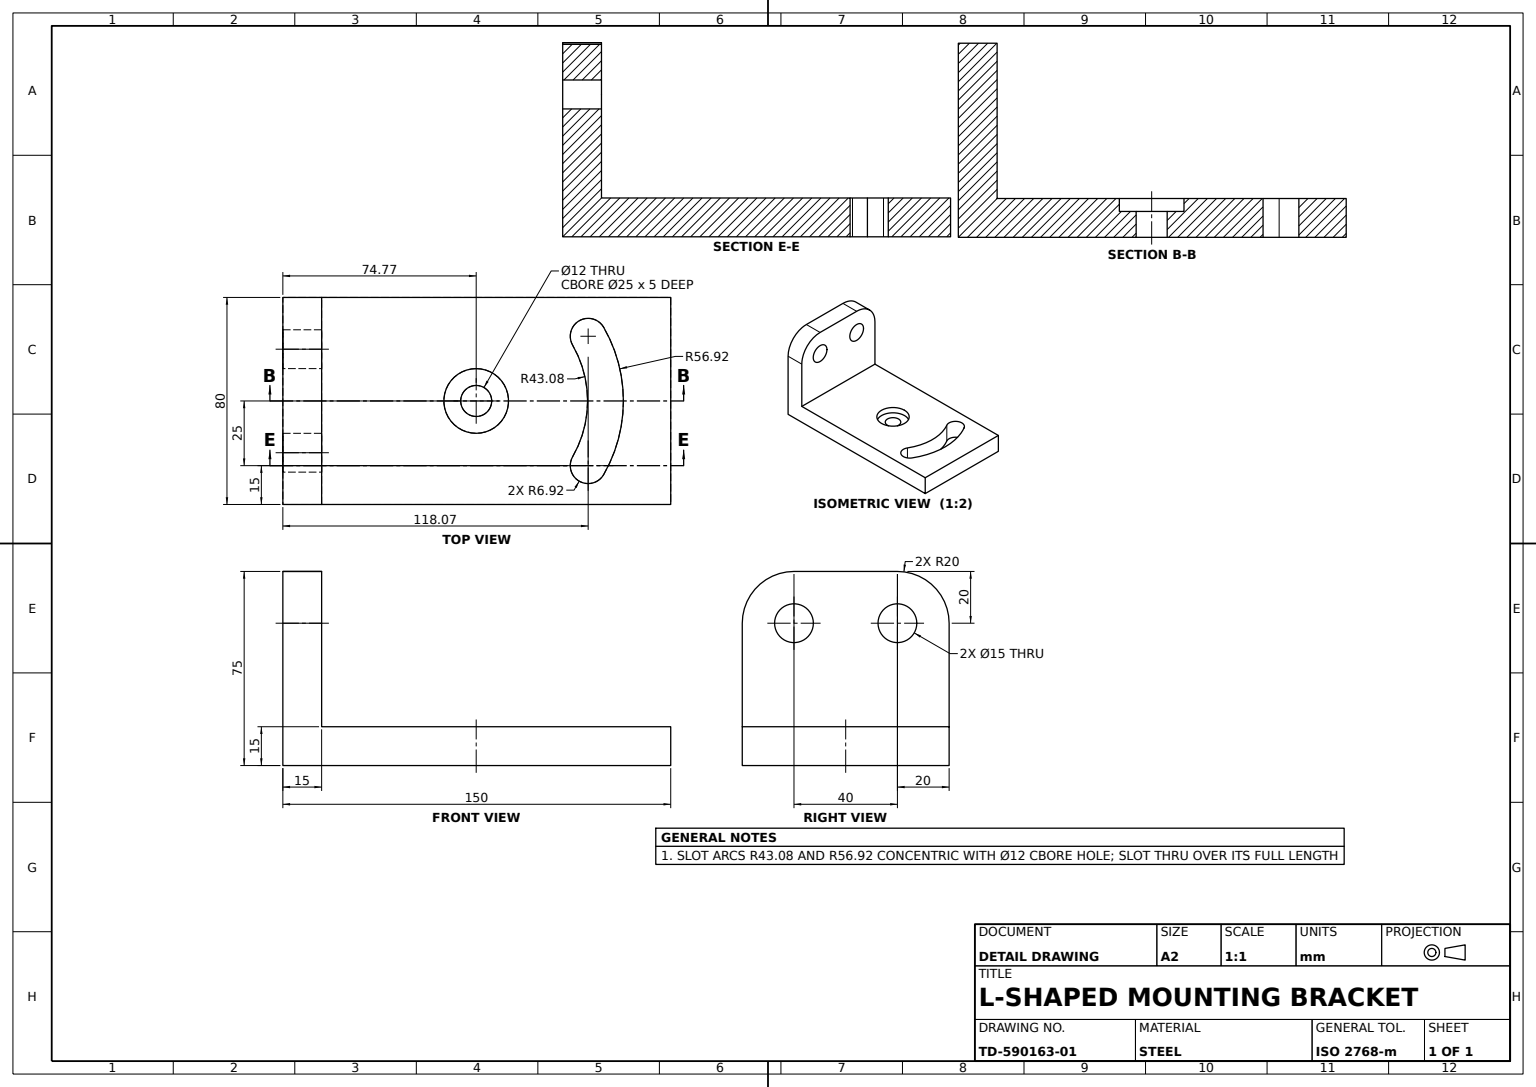
from build123d import *

# Parameters (mm, degrees)
BASE_PLATE_SKETCH_W             = 150
BASE_PLATE_SKETCH_H             = 80
BASE_PLATE_SKETCH_R             = 12.5
BASE_PLATE_DEPTH                = 15
SKETCH1_4_R                     = 12.5
SKETCH1_4_R_2                   = 6
BASE_CONTOUR_EXTRUDE_10MM_DEPTH = 10
UPRIGHT_WALL_SKETCH_W           = 15
UPRIGHT_WALL_SKETCH_H           = 80
UPRIGHT_WALL_DEPTH              = 60
UPRIGHT_TOP_FILLET_R20_R        = 20
UPRIGHT_HOLES_SKETCH_R          = 7.5
UPRIGHT_MOUNTING_HOLES_DEPTH    = 40


with BuildPart() as part:
    # Base Plate Sketch → Base Plate (new body)
    with BuildSketch(Plane(origin=(0, 0, 0), x_dir=(1, 0, 0), z_dir=(0, 1, 0))):
        with Locations((75, 0)):
            Rectangle(BASE_PLATE_SKETCH_W, BASE_PLATE_SKETCH_H)
        with Locations(Location((74.768392371, 0, 0), (0, 0, 270))):
            Circle(BASE_PLATE_SKETCH_R, mode=Mode.SUBTRACT)
        with BuildLine():
            ThreePointArc((124.066474122, 28.46226077), (114.60740179, 30.996811562), (112.072850998, 21.53773923))
            ThreePointArc((112.072850998, 21.53773923), (117.843870831, 0), (112.072850998, -21.53773923))
            ThreePointArc((112.072850998, -21.53773923), (114.60740179, -30.996811562), (124.066474122, -28.46226077))
            ThreePointArc((124.066474122, -28.46226077), (131.69291391, 0), (124.066474122, 28.46226077))
        make_face(mode=Mode.SUBTRACT)
    extrude(amount=BASE_PLATE_DEPTH)

    # Sketch1_4 → Base Contour Extrude 10mm (add)
    with BuildSketch(Plane(origin=(0, 0, 0), x_dir=(1, 0, 0), z_dir=(0, 1, 0))):
        with Locations(Location((74.768392371, 0, 0), (0, 0, 270))):
            Circle(SKETCH1_4_R)
        with Locations(Location((74.768392371, 0, 0), (0, 0, 270))):
            Circle(SKETCH1_4_R_2, mode=Mode.SUBTRACT)
    extrude(amount=BASE_CONTOUR_EXTRUDE_10MM_DEPTH)

    # Upright Wall Sketch → Upright Wall (add)
    with BuildSketch(Plane(origin=(0, 15, 0), x_dir=(1, 0, 0), z_dir=(0, 1, 0))):
        with Locations((7.5, 0)):
            Rectangle(UPRIGHT_WALL_SKETCH_W, UPRIGHT_WALL_SKETCH_H)
    extrude(amount=UPRIGHT_WALL_DEPTH)

    # Upright Top Fillet R20
    upright_top_fillet_r20_edges = [part.edges().sort_by_distance(p)[0] for p in [
        (7.5, 75, 40),
        (7.5, 75, -40),
    ]]
    fillet(upright_top_fillet_r20_edges, radius=UPRIGHT_TOP_FILLET_R20_R)

    # Upright Holes Sketch → Upright Mounting Holes (cut, symmetric)
    with BuildSketch(Plane(origin=(15, 0, 0), x_dir=(0, 0, -1), z_dir=(1, 0, 0))):
        with Locations((20, 55)):
            Circle(UPRIGHT_HOLES_SKETCH_R)
        with Locations((-20, 55)):
            Circle(UPRIGHT_HOLES_SKETCH_R)
    extrude(amount=UPRIGHT_MOUNTING_HOLES_DEPTH, both=True, mode=Mode.SUBTRACT)


solid = part.part
